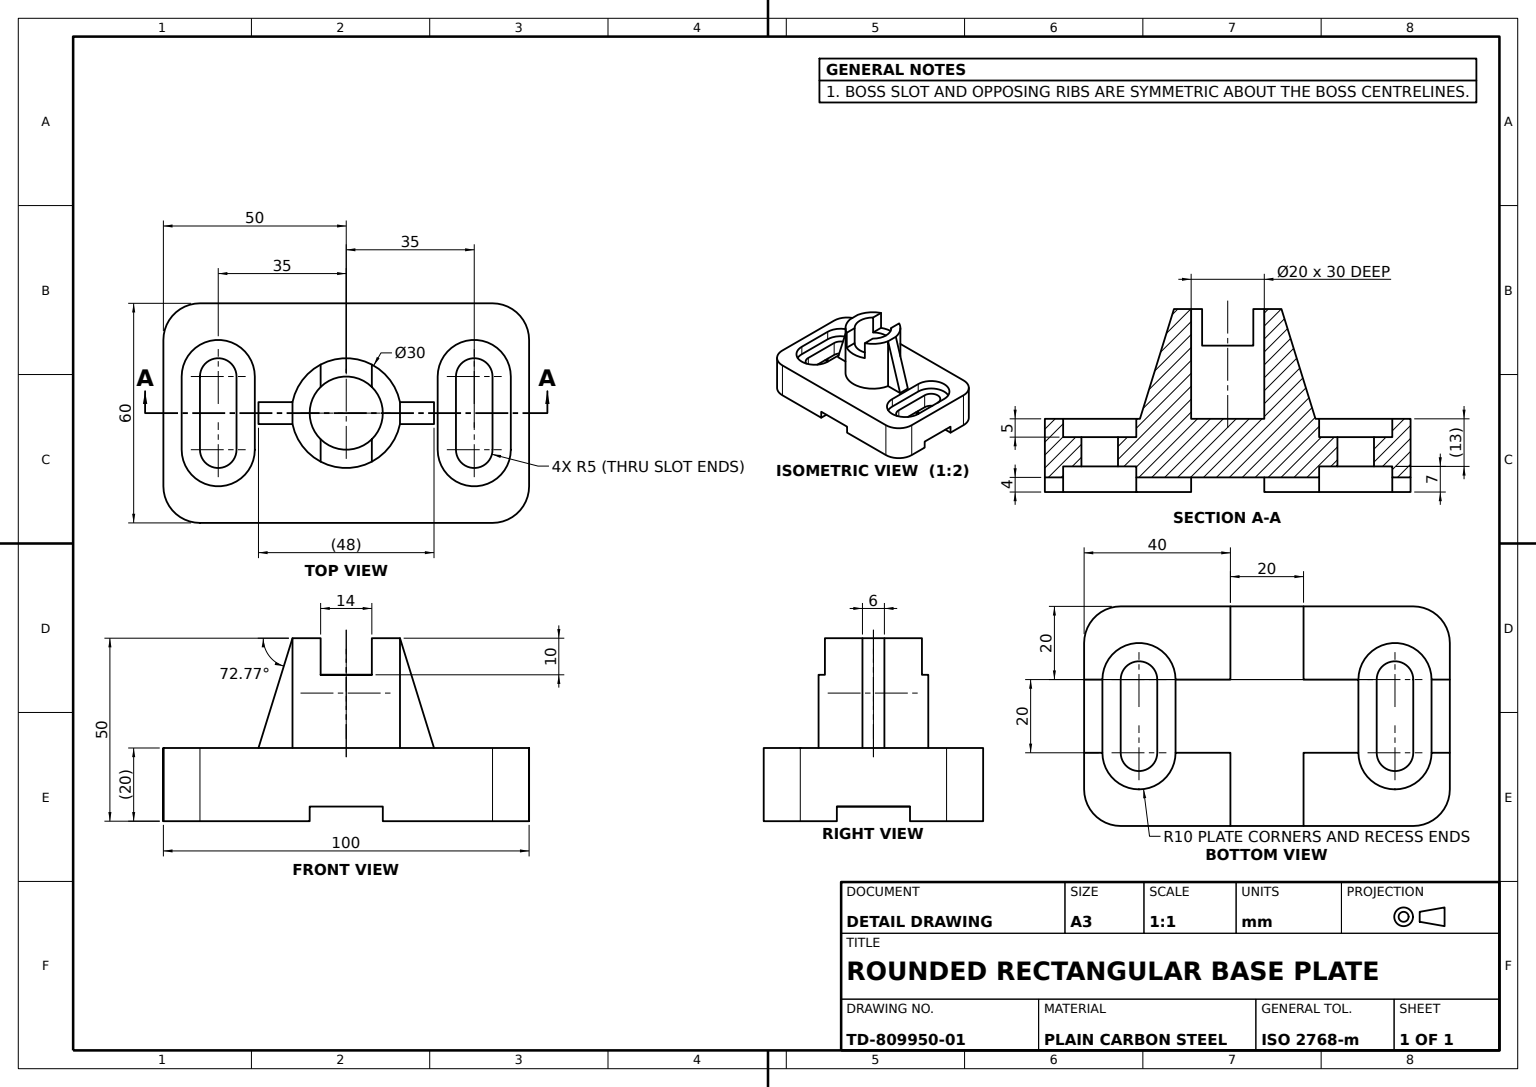
SolidWorks part; units mm, degrees
material "Plain Carbon Steel"
ref_plane "Front Plane" through (0, 0, 0) normal (0, 0, 1) x (1, 0, 0)
ref_plane "Top Plane" through (0, 0, 0) normal (0, 1, 0) x (1, 0, 0)
ref_plane "Right Plane" through (0, 0, 0) normal (1, 0, 0) x (0, 0, -1)
sketch "Base Plate Profile Sketch" plane through (0, 0, 0) normal (0, 0, 1) x (1, 0, 0)
  line L1 (-10, 4) -> (10, 4)
  line L2 (10, 4) -> (10, 0)
  line L3 (10, 0) -> (50, 0)
  line L4 (50, 0) -> (50, 20)
  line L5 (50, 20) -> (-50, 20)
  line L6 (0, 0) -> (0, 29.7963) construction
  line L7 (-50, 0) -> (-50, 20)
  line L8 (-10, 0) -> (-50, 0)
  line L9 (-10, 4) -> (-10, 0)
  dimension "D1" = 4
  dimension "D2" = 20
  dimension "D3" = 20
  dimension "D4" = 100
extrude "Base Plate" add sketch "Base Plate Profile Sketch" along normal mid plane 60
sketch "Underside Notches Sketch" plane through (0, 20, 0) normal (0, 1, 0) x (1, 0, 0)
  line L0 (40, 30) -> (50, 30)
  line L1 (-12.2356, 0) -> (16.276, 0) construction
  line L2 (50, 30) -> (50, 20)
  line L4 (0, 13.7989) -> (0, -10.6634) construction
  line L5 (-50, 30) -> (-50, 20)
  line L6 (-40, 30) -> (-50, 30)
  line L7 (-50, -30) -> (-50, -20)
  line L8 (-40, -30) -> (-50, -30)
  line L9 (50, -30) -> (50, -20)
  line L10 (40, -30) -> (50, -30)
  arc A0 (50, 20) -> (40, 30) centre (40, 20) ccw
  arc A1 (-50, 20) -> (-40, 30) centre (-40, 20) cw
  arc A2 (-50, -20) -> (-40, -30) centre (-40, -20) ccw
  arc A3 (50, -20) -> (40, -30) centre (40, -20) cw
  dimension "D1" = 10
  dimension "D2" = 10
extrude "Underside Notches" cut sketch "Underside Notches Sketch" against normal blind 60
sketch "Pivot Boss Sketch" plane through (0, 20, 0) normal (0, 1, 0) x (1, 0, 0)
  circle A0 centre (0, 0) radius 15
  circle A1 centre (0, 0) radius 10
  dimension "D1" = 30
  dimension "D2" = 20
extrude "Pivot Boss Ø30" add sketch "Pivot Boss Sketch" along normal blind 30
sketch "Slot Recess A Sketch" plane through (0, 20, 0) normal (0, 1, 0) x (1, 0, 0)
  line L0 (0, 0) -> (35, 0) construction
  line L1 (35, -10) -> (35, 10) construction
  line L2 (30, -10) -> (30, 10)
  line L3 (40, -10) -> (40, 10)
  line L4 (-35, -10) -> (-35, 10) construction
  line L7 (0, 0) -> (0, -21.2593) construction
  line L8 (-30, -10) -> (-30, 10)
  line L9 (-40, -10) -> (-40, 10)
  arc A0 (30, -10) -> (40, -10) centre (35, -10) ccw
  arc A1 (40, 10) -> (30, 10) centre (35, 10) ccw
  arc A4 (-30, -10) -> (-40, -10) centre (-35, -10) cw
  arc A5 (-40, 10) -> (-30, 10) centre (-35, 10) cw
  point P5 (35, 0)
  point P12 (-35, 0)
  dimension "D1" = 20
  dimension "D2" = 10
  dimension "D4" = 35
extrude "Slot Recess A" cut sketch "Slot Recess A Sketch" against normal blind 13
sketch "Slot Inner Cut A Sketch" plane through (0, 20, 0) normal (0, 1, 0) x (1, 0, 0)
  line L0 (35, -10) -> (35, 10) construction
  line L1 (25, -10) -> (25, 10)
  line L2 (45, -10) -> (45, 10)
  line L3 (0, 0) -> (0, 21.986) construction
  line L4 (-35, -10) -> (-35, 10) construction
  line L5 (-25, -10) -> (-25, 10)
  line L6 (-45, -10) -> (-45, 10)
  arc A0 (25, -10) -> (45, -10) centre (35, -10) ccw
  arc A1 (45, 10) -> (25, 10) centre (35, 10) ccw
  arc A2 (-25, -10) -> (-45, -10) centre (-35, -10) cw
  arc A3 (-45, 10) -> (-25, 10) centre (-35, 10) cw
  point P2 (35, 0)
  point P13 (-35, 0)
  dimension "D1" = 20
  dimension "D2" = 20
extrude "Slot Inner Cut A" cut sketch "Slot Inner Cut A Sketch" against normal blind 5
sketch "Slot Recess B Sketch" plane through (0, 0, 0) normal (0, -1, 0) x (1, 0, 0)
  line L0 (0, 0) -> (35, 0) construction
  line L1 (35, 10) -> (35, -10) construction
  line L2 (45, 10) -> (45, -10)
  line L3 (25, 10) -> (25, -10)
  line L4 (0, 0) -> (0, -17.7938) construction
  line L5 (-35, 10) -> (-35, -10) construction
  line L6 (-45, 10) -> (-45, -10)
  line L7 (-25, 10) -> (-25, -10)
  arc A0 (45, 10) -> (25, 10) centre (35, 10) ccw
  arc A1 (25, -10) -> (45, -10) centre (35, -10) ccw
  arc A2 (-45, 10) -> (-25, 10) centre (-35, 10) cw
  arc A3 (-25, -10) -> (-45, -10) centre (-35, -10) cw
  point P5 (35, 0)
  point P13 (-35, 0)
  dimension "D1" = 35
  dimension "D2" = 20
  dimension "D3" = 20
extrude "Slot Recess B" cut sketch "Slot Recess B Sketch" against normal blind 7
sketch "Slot Inner Cut B Sketch" plane through (50, 0, 0) normal (1, 0, 0) x (0, 0, -1)
  line L1 (0, 4) -> (10, 4)
  line L2 (10, 4) -> (10, 0)
  line L3 (10, 0) -> (-10, 0)
  line L4 (-20, 0) -> (20, 0) construction
  line L5 (-10, 0) -> (-10, 4)
  line L6 (-10, 4) -> (0, 4)
  dimension "D1" = 10
  dimension "D2" = 4
  dimension "D3" = 4
extrude "Slot Inner Cut B" cut sketch "Slot Inner Cut B Sketch" against normal through all
sketch "Boss Slot Sketch" plane through (0, 0, 0) normal (0, 0, 1) x (1, 0, 0)
  line L0 (0, 50) -> (7, 50)
  line L1 (15, 50) -> (-15, 50) construction
  line L2 (10, 50) -> (-10, 50) construction
  line L3 (7, 50) -> (7, 40)
  line L4 (7, 40) -> (-7, 40)
  line L5 (-7, 40) -> (-7, 50)
  line L6 (-7, 50) -> (0, 50)
  dimension "D1" = 14
  dimension "D2" = 10
  dimension "D3" = 7
extrude "Boss Slot Cut" cut sketch "Boss Slot Sketch" against normal through all both and the other way through all
sketch "Support Rib Sketch" plane through (0, 0, 0) normal (1, 0, 0) x (0, 0, -1)
  line L1 (-20, 20) -> (20, 20) construction
  line L2 (13.2665, 50) -> (-13.2665, 50) construction
  line L3 (0, 50) -> (3, 50)
  line L4 (3, 50) -> (3, 20)
  line L5 (3, 20) -> (-3, 20)
  line L6 (-3, 20) -> (-3, 50)
  line L7 (-3, 50) -> (0, 50)
  dimension "D1" = 6
  dimension "D2" = 3
extrude "Support Rib" add sketch "Support Rib Sketch" along normal mid plane 48
sketch "Rib Trim Sketch" plane through (0, 0, 0) normal (0, 0, 1) x (1, 0, 0)
  line L0 (0, 20) -> (0, 52.5766) construction
  line L1 (40, 20) -> (-40, 20) construction
  line L2 (24, 50) -> (24, 20) construction
  line L3 (24, 20) -> (14.6969, 50)
  line L4 (14.6969, 50) -> (24, 50)
  line L5 (24, 50) -> (24, 20)
  line L6 (-24, 50) -> (-24, 20)
  line L7 (-14.6969, 50) -> (-24, 50)
  line L8 (-24, 20) -> (-14.6969, 50)
extrude "Rib Trim Cut" cut sketch "Rib Trim Sketch" against normal through all both and the other way through all
sketch "Pivot Bore Sketch" plane through (0, 20, 0) normal (0, 1, 0) x (1, 0, 0)
  circle A0 centre (0, 0) radius 10
  dimension "D1" = 20
extrude "Pivot Bore Ø20" cut sketch "Pivot Bore Sketch" along normal blind 48
